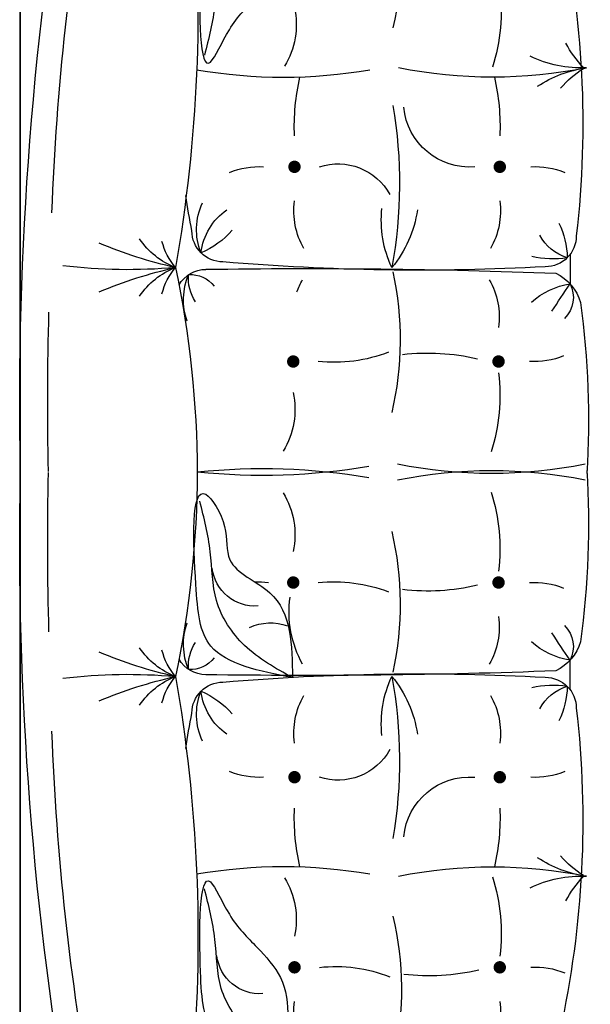
# Model space of a CAD drawing. Units: inches. Extents: x 844 to 2234, y 346 to 1084.
# Tile 51 of 93: x 1843 to 1858, y 688 to 713. Entities that reach past the tile are written whole.
import ezdxf

# ---------------------------------------------------------------- set-up
doc = ezdxf.new("R2010")
doc.units = ezdxf.units.IN
doc.header["$MEASUREMENT"] = 0
doc.layers.add('A-WALL', color=7, linetype='Continuous', lineweight=35)
doc.layers.add('furniture', color=8, linetype='Continuous', lineweight=18)
doc.layers.add('RA-AP-01$0$FURN', color=3, linetype='Continuous')
doc.layers.add('RA-AP-01$0$WOOD', color=64, linetype='Continuous')

# ---------------------------------------------------------------- blocks, each defined once
blk = doc.blocks.new('A$C7EE91E48')
at = {"layer": 'RA-AP-01$0$FURN'}
for p, q in [((8.4752, -8.8836), (8.5044, -8.8836)), ((8.5044, -8.8836), (8.5227, -8.8836)), ((9.1476, -8.8836), (9.1292, -8.8836)), ((9.1768, -8.8836), (9.1476, -8.8836))]:
    blk.add_line(p, q, dxfattribs=at)
at = {"layer": 'RA-AP-01$0$FURN', "const_width": 0.01}
for points in [[(8.0279, -9.0019, -1), (8.0279, -8.9919, -1)], [(8.3342, -9.0019, 1), (8.3342, -8.9919, 1)], [(8.6479, -9.0039, -1), (8.6479, -8.9939, -1)], [(9.004, -9.0039, 1), (9.004, -8.9939, 1)], [(9.3177, -9.0019, -1), (9.3177, -8.9919, -1)], [(8.0279, -9.3223, 1), (8.0279, -9.3323, 1)], [(8.3342, -9.3223, -1), (8.3342, -9.3323, -1)], [(8.6479, -9.3243, 1), (8.6479, -9.3343, 1)], [(9.004, -9.3243, -1), (9.004, -9.3343, -1)], [(9.3177, -9.3223, 1), (9.3177, -9.3323, 1)]]:
    blk.add_lwpolyline(points, format="xyb", close=True, dxfattribs=at)
at = {"layer": 'RA-AP-01$0$FURN'}
for centre, radius, start, end in [((8.2641, -10.4424), 1.5791, 83.4116, 102.408), ((8.0633, -8.7497), 0.1579, 296.9155, 314.5948), ((7.9834, -8.8653), 0.1916, 334.4169, 2.4147), ((7.4244, -9.0082), 0.7655, 348.5826, 11.3727), ((8.3595, -8.8326), 0.1864, 187.6182, 213.7074), ((8.3098, -8.7788), 0.1579, 211.9342, 229.6135), ((8.5734, -8.9396), 0.0754, 106.0166, 154.1254), ((8.744, -10.2748), 1.4207, 86.5948, 97.7424), ((8.0629, -9.0102), 0.7655, 348.5826, 11.3727), ((8.9079, -10.2748), 1.4207, 82.2576, 93.4052), ((9.589, -9.0102), 0.7655, 168.6273, 191.4174), ((9.0785, -8.9396), 0.0754, 25.8746, 73.9834), ((9.3879, -10.4424), 1.5791, 77.592, 96.5884), ((9.3421, -8.7788), 0.1579, 310.3865, 328.0658), ((9.2924, -8.8326), 0.1864, 326.2926, 352.3818), ((10.2276, -9.0082), 0.7655, 168.6273, 191.4174), ((9.6686, -8.8653), 0.1916, 177.5853, 205.5831), ((9.5886, -8.7497), 0.1579, 225.4052, 243.0845), ((8.4452, -8.9237), 0.05, 0, 90), ((8.5446, -8.9264), 0.0479, 44.5975, 117.1929), ((8.6431, -8.8646), 0.1219, 188.9538, 221.9624), ((9.1542, -7.9707), 1.1102, 235.3335, 238.0671), ((9.1073, -8.9264), 0.0479, 62.8071, 135.4025), ((8.4977, -7.9707), 1.1102, 301.9329, 304.6665), ((9.0089, -8.8646), 0.1219, 318.0376, 351.0462), ((9.2067, -8.9237), 0.05, 90, 180), ((7.9069, -8.939), 0.1213, 356.2685, 22.6624), ((8.4553, -8.939), 0.1213, 157.3376, 183.7315), ((8.4834, -9.0206), 0.1324, 91.1993, 116.1112), ((8.411, -8.8679), 0.0726, 297.3225, 343.6441), ((8.3504, -8.912), 0.1324, 345.3922, 10.3041), ((8.5269, -8.941), 0.1213, 356.2685, 22.6624), ((9.1251, -8.941), 0.1213, 157.3376, 183.7315), ((9.3016, -8.912), 0.1324, 169.6959, 194.6078), ((9.1686, -9.0206), 0.1324, 63.8888, 88.8007), ((9.241, -8.8679), 0.0726, 196.3559, 242.6775), ((9.1967, -8.939), 0.1213, 356.2685, 22.6624), ((19.2274, -9.306), 10.7293, 177.86728, 180.87576), ((-1.5755, -9.306), 10.7293, 359.12424, 2.13272), ((4.8029, -9.1271), 3.698, 355.1082, 3.1536), ((12.8491, -9.1271), 3.698, 176.8464, 184.8918), ((8.0823, -9.2969), 0.3024, 72.4119, 96.9055), ((9.5696, -9.2969), 0.3024, 83.0945, 107.5881), ((7.9567, -9.1172), 0.1214, 82.3083, 119.8581), ((8.2692, -9.3452), 0.3487, 87.5342, 103.1608), ((8.4055, -9.1172), 0.1214, 60.1419, 97.6917), ((8.5767, -9.1192), 0.1214, 82.3083, 119.8581), ((8.7023, -9.299), 0.3024, 72.4119, 96.9055), ((8.9496, -9.299), 0.3024, 83.0945, 107.5881), ((9.0753, -9.1192), 0.1214, 60.1419, 97.6917), ((9.2465, -9.1172), 0.1214, 82.3083, 119.8581), ((9.3827, -9.3452), 0.3487, 76.8392, 92.4658), ((8.3659, -9.111), 0.3517, 166.8325, 186.5875), ((8.2285, -9.0458), 0.106, 275.1859, 4.8073), ((8.9859, -9.113), 0.3517, 166.8325, 186.5875), ((8.666, -9.113), 0.3517, 353.4125, 13.1675), ((9.4234, -9.0458), 0.106, 175.1927, 264.8141), ((8.378, -9.3133), 0.1855, 50.3168, 82.0523), ((9.2739, -9.3133), 0.1855, 97.9477, 129.6832), ((7.9929, -9.6653), 0.5101, 76.6878, 102.3818), ((8.3614, -9.9068), 0.7485, 79.6011, 99.6906), ((8.6129, -9.6673), 0.5101, 76.6878, 102.3818), ((9.0391, -9.6673), 0.5101, 77.6182, 103.3122), ((9.2906, -9.9068), 0.7485, 80.3094, 100.3989), ((9.6591, -9.6653), 0.5101, 77.6182, 103.3122), ((7.785, -9.2618), 0.2442, 354.0076, 21.0983), ((8.4248, -9.2574), 0.0954, 118.8034, 198.2253), ((8.4207, -9.0107), 0.1769, 263.6796, 295.3608), ((8.405, -9.2638), 0.2442, 354.0076, 21.0983), ((9.2469, -9.2638), 0.2442, 158.9017, 185.9924), ((9.2312, -9.0107), 0.1769, 244.6392, 276.3204), ((9.2271, -9.2574), 0.0954, 341.7747, 61.1966), ((7.367, -9.3453), 0.8233, 350.2449, 9.7551), ((7.8327, -9.3782), 0.9989, 353.9343, 9.823), ((9.8193, -9.3782), 0.9989, 170.177, 186.0657), ((10.285, -9.3453), 0.8233, 170.2449, 189.7551), ((7.9567, -9.2069), 0.1214, 240.1419, 277.6917), ((8.4055, -9.2069), 0.1214, 262.3083, 299.8581), ((9.2465, -9.2069), 0.1214, 240.1419, 277.6917), ((8.1048, -9.4539), 0.1295, 58.6204, 102.0099), ((8.2692, -8.9789), 0.3487, 256.8392, 272.4658), ((8.6002, -9.1634), 0.1726, 240.9024, 278.0073), ((8.7248, -9.456), 0.1295, 58.6204, 102.0099), ((8.9271, -9.456), 0.1295, 77.9901, 121.3796), ((9.0753, -9.209), 0.1214, 289.6086, 299.8581), ((9.3827, -8.9789), 0.3487, 267.5342, 283.1608), ((9.5471, -9.4539), 0.1295, 77.9901, 121.3796), ((8.5004, -9.3657), 0.0825, 335.8161, 19.2747), ((8.405, -9.3948), 0.2442, 0.7304, 5.9924), ((8.0543, -9.3837), 0.0689, 175.5384, 263.5805), ((8.4553, -9.3851), 0.1213, 176.2685, 202.6624), ((8.6789, -9.3912), 0.0689, 175.5384, 263.5805), ((9.1967, -9.3851), 0.1213, 337.3376, 3.7315), ((8.4847, -9.3794), 0.0991, 214.8912, 263.0774), ((8.3451, -9.5317), 0.1386, 22.9132, 48.7711), ((9.3068, -9.5317), 0.1386, 131.2289, 157.0868), ((9.1673, -9.3794), 0.0991, 276.9226, 325.1088), ((8.4374, -9.4424), 0.05, 270, 0), ((9.2146, -9.4424), 0.05, 180, 270), ((8.5494, -9.4699), 0.05, 180, 239.8522), ((8.5556, -9.4948), 0.0479, 127.3166, 183.4247), ((9.0963, -9.4948), 0.0479, 356.5753, 52.6834), ((9.1025, -9.4699), 0.05, 300.1478, 360), ((8.0772, -11.9348), 2.4522, 80.1542, 94.8039), ((8.4354, -9.3857), 0.0993, 244.3656, 292.0953), ((8.8331, -11.1187), 1.6349, 90.2483, 101.88), ((8.514, -9.4297), 0.0683, 264.7816, 303.327), ((8.8189, -11.1187), 1.6349, 78.12, 89.7517), ((9.1379, -9.4297), 0.0683, 236.673, 275.2184), ((9.5748, -11.9348), 2.4522, 85.1961, 99.8458), ((9.2166, -9.3857), 0.0993, 247.9047, 295.6344), ((8.1811, -8.1864), 1.3309, 278.6229, 281.1036), ((8.5483, -9.4017), 0.1042, 247.1307, 289.5172), ((9.1036, -9.4017), 0.1042, 250.4828, 292.8693), ((9.4709, -8.1864), 1.3309, 258.8964, 261.3771), ((8.3825, -9.4751), 0.122, 303.7136, 339.041), ((8.4279, -9.4377), 0.1062, 284.3648, 310.2303), ((7.8141, -9.3689), 0.6986, 337.0091, 347.612), ((7.6413, -9.5958), 0.8587, 353.0376, 5.1445), ((8.6105, -9.4751), 0.122, 200.959, 236.2864), ((8.5651, -9.4377), 0.1062, 229.7697, 255.6352), ((9.1788, -9.3689), 0.6986, 192.388, 202.9909), ((9.0415, -9.4751), 0.122, 303.7136, 339.041), ((9.0869, -9.4377), 0.1062, 284.3648, 310.2303), ((8.4731, -9.3689), 0.6986, 337.0091, 347.612), ((10.0107, -9.5958), 0.8587, 174.8555, 186.9624), ((9.2694, -9.4751), 0.122, 200.959, 236.2864), ((9.224, -9.4377), 0.1062, 229.7697, 255.6352), ((9.8378, -9.3689), 0.6986, 192.388, 202.9909), ((8.5724, -5.4361), 4.2848, 259.7801, 267.8084), ((9.0796, -5.4361), 4.2848, 272.1916, 280.2199), ((8.7159, -4.2841), 5.4854, 259.9939, 271.1496), ((8.936, -4.2841), 5.4854, 268.8504, 280.0061), ((8.7159, -4.2841), 5.4404, 268.4485, 271.1496), ((8.936, -4.2841), 5.4404, 268.8504, 271.5515)]:
    blk.add_arc(centre, radius, start, end, dxfattribs=at)
for points, knots in [([(7.8747, -9.3485), (7.9231, -9.3393), (7.9933, -9.326), (8.0638, -9.3901), (8.1031, -9.4315), (8.221, -9.4812), (8.0194, -9.4811), (7.9064, -9.4702), (7.8857, -9.3906), (7.8747, -9.3485)], [0, 0, 0, 0, 0.1367587, 0.1981302, 0.267773, 0.3281195, 0.4737578, 0.5765194, 0.6920332, 0.6920332, 0.6920332, 0.6920332]), ([(8.4947, -9.3305), (8.5098, -9.3579), (8.5387, -9.4102), (8.6151, -9.4603), (8.6994, -9.4595), (8.7521, -9.4728), (8.7791, -9.4797)], [0, 0, 0, 0, 0.0929945, 0.178054, 0.2574251, 0.3407808, 0.3407808, 0.3407808, 0.3407808]), ([(8.4947, -9.3305), (8.547, -9.3311), (8.63, -9.3319), (8.67, -9.4425), (8.7389, -9.4316), (8.8424, -9.4963), (8.6448, -9.4874), (8.5233, -9.4759), (8.5051, -9.3838), (8.4947, -9.3305)], [0, 0, 0, 0, 0.1415752, 0.2249019, 0.2789443, 0.3392908, 0.4849291, 0.5876907, 0.7285367, 0.7285367, 0.7285367, 0.7285367]), ([(9.7773, -9.3485), (9.7288, -9.3393), (9.6586, -9.326), (9.5882, -9.3901), (9.5488, -9.4315), (9.4309, -9.4812), (9.6325, -9.4811), (9.7455, -9.4702), (9.7663, -9.3906), (9.7773, -9.3485)], [0, 0, 0, 0, 0.1367587, 0.1981302, 0.267773, 0.3281195, 0.4737578, 0.5765194, 0.6920332, 0.6920332, 0.6920332, 0.6920332]), ([(7.8747, -9.3485), (7.8896, -9.3663), (7.9228, -9.4056), (7.9899, -9.4532), (8.0749, -9.4519), (8.1275, -9.4653), (8.1544, -9.4722)], [0, 0, 0, 0, 0.0700185, 0.155078, 0.2344492, 0.3178049, 0.3178049, 0.3178049, 0.3178049]), ([(9.7773, -9.3485), (9.7623, -9.3663), (9.7292, -9.4056), (9.662, -9.4532), (9.577, -9.4519), (9.5245, -9.4653), (9.4975, -9.4722)], [0, 0, 0, 0, 0.0700185, 0.155078, 0.2344492, 0.3178049, 0.3178049, 0.3178049, 0.3178049])]:
    blk.add_open_spline(points, degree=3, knots=knots, dxfattribs=at)
blk = doc.blocks.new('A$C5D2F253E')
at = {"layer": 'RA-AP-01$0$WOOD', "xscale": -1, "rotation": 180}
blk.add_blockref('A$C7EE91E48', (-8.833, -7.2888), dxfattribs=at)

msp = doc.modelspace()

# ---------------------------------------------------------------- linework, layer by layer
at = {"layer": 'A-WALL'}
msp.add_line((1843.099, 766.455), (1843.099, 629.455), dxfattribs=at)

# ---------------------------------------------------------------- block references
at = {"layer": 'furniture', "xscale": 15.94108302203742, "yscale": 15.94108302203742, "zscale": 15.94108302203742, "rotation": 90}
msp.add_blockref('A$C5D2F253E', (1882.631, 701.403), dxfattribs=at)

doc.saveas('drawing.dxf')
